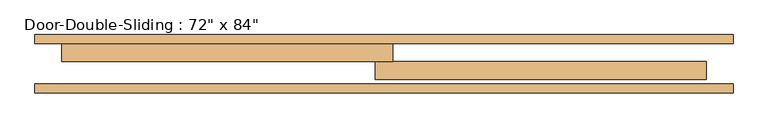
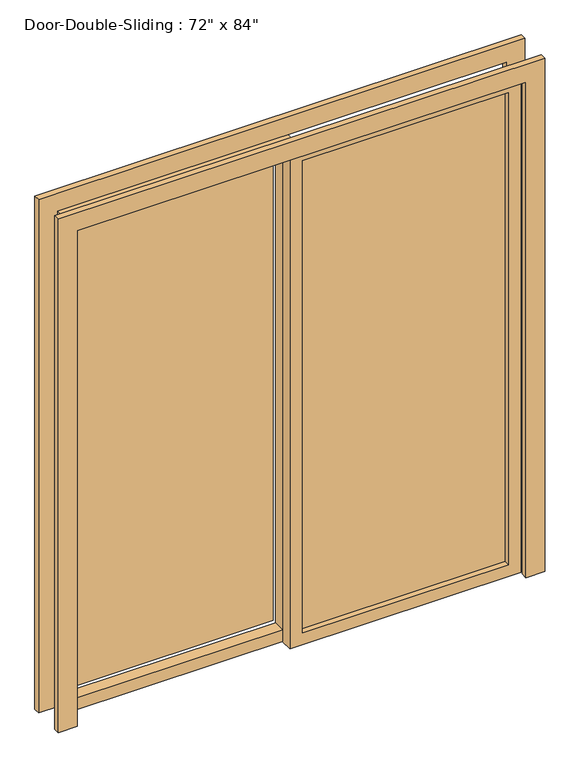
"""IFC4 building model written with IfcOpenShell, lengths in millimetres: door geometry."""

from ifc_helpers import new_model, si_unit, frame, origin, place, context, project, spatial, polyline, outline, extrude, source, transform, mapped, element, save


def door_166d4031(model_context):
    return source(origin(), model_context, "Body", "SweptSolid", [
        extrude(outline(polyline([(0.0, 990.6), (2209.8, 990.6), (2209.8, -990.6), (0.0, -990.6), (0.0, -914.4), (2133.6, -914.4), (2133.6, 914.4), (0.0, 914.4), (0.0, 990.6)])), frame((0.0, 184.15, 0.0), z_axis=(0.0, 1.0, 0.0), x_axis=(0.0, 0.0, 1.0)), (0.0, 0.0, 1.0), 25.4),
        extrude(outline(polyline([(0.0, -990.6), (0.0, -914.4), (2133.6, -914.4), (2133.6, 914.4), (0.0, 914.4), (0.0, 990.6), (2209.8, 990.6), (2209.8, -990.6), (0.0, -990.6)])), frame((0.0, 44.45, 0.0), z_axis=(0.0, 1.0, 0.0), x_axis=(0.0, 0.0, 1.0)), (0.0, 0.0, 1.0), 25.4),
        extrude(outline(polyline([(2133.6, 25.4), (2133.6, -914.4), (0.0, -914.4), (0.0, 25.4), (2133.6, 25.4)]), holes=[polyline([(2082.8, -25.4), (50.8, -25.4), (50.8, -863.6), (2082.8, -863.6), (2082.8, -25.4)])]), frame((0.0, 133.35, 0.0), z_axis=(0.0, 1.0, 0.0), x_axis=(0.0, 0.0, 1.0)), (0.0, 0.0, 1.0), 50.8),
        extrude(outline(polyline([(2133.6, -25.4), (0.0, -25.4), (0.0, 914.4), (2133.6, 914.4), (2133.6, -25.4)]), holes=[polyline([(2082.8, 25.4), (2082.8, 863.6), (50.8, 863.6), (50.8, 25.4), (2082.8, 25.4)])]), frame((0.0, 82.55, 0.0), z_axis=(0.0, 1.0, 0.0), x_axis=(0.0, 0.0, 1.0)), (0.0, 0.0, 1.0), 50.8),
        extrude(outline(polyline([(-25.4, 200.025), (-863.6, 200.025), (-863.6, 206.375), (-25.4, 206.375), (-25.4, 200.025)])), frame((0.0, 0.0, 50.8), z_axis=(0.0, 0.0, 1.0), x_axis=(1.0, 0.0, 0.0)), (0.0, 0.0, 1.0), 2032.0),
        extrude(outline(polyline([(25.4, 111.125), (863.6, 111.125), (863.6, 104.775), (25.4, 104.775), (25.4, 111.125)])), frame((0.0, 0.0, 50.8), z_axis=(0.0, 0.0, 1.0), x_axis=(1.0, 0.0, 0.0)), (0.0, 0.0, 1.0), 2032.0),
    ])


if __name__ == "__main__":
    model = new_model("IFC4")
    model_context = context("Model", 3, world=origin())
    ifc_project = project(units=[si_unit("LENGTHUNIT", "METRE", prefix="MILLI")], contexts=[model_context])
    site = spatial("IfcSite", under=ifc_project)
    building = spatial("IfcBuilding", under=site)
    placement = place(None, origin())
    door_shape = door_166d4031(model_context)
    element("IfcDoor", 1, ObjectType="Door-Double-Sliding : 72\" x 84\"", at=placement, inside=building, context=model_context, shape_type="MappedRepresentation", body=[
        mapped(door_shape, transform((0.0, 0.0, 0.0), x_axis=(1.0, 0.0, 0.0), y_axis=(0.0, 1.0, 0.0), z_axis=(0.0, 0.0, 1.0))),
    ])
    save(model, "model.ifc")

# Revit data of these elements
# Type "Door-Double-Sliding : 72\" x 84\""
#   Type Mark = "12"
#   Construction Type Id = "opn-d45"
#   Assembly Code = "C1020"
#   Analytic Construction = "Wood frame, double glass door "
#   Thickness = 0' - 2"
#   Thermal Resistance (R) = 1.8150 (h·ft²·°F)/BTU
#   Heat Transfer Coefficient (U) = 0.5510 BTU/(h·ft²·°F)
#   Height = 7' - 0"
#   Rail Width = 0' - 2"
#   Stiles = 0' - 2"
#   Trim Projection Ext = 0' - 1"
#   Trim Projection Int = 0' - 1"
#   Trim Width = 0' - 3"
#   Width = 6' - 0"
#   Define Thermal Properties by = 1
#   Glazing = Glass
#   Panel Material = Wood - Birch - Solid Stained Light Low Gloss
#   Trim Material = Paint - Sienna
#   Visual Light Transmittance = 0
#   Solar Heat Gain Coefficient = 0
#   Function = (empty or 0)
#   Wall Closure = (empty or 0)
# Element 1 (IfcDoor, "Door-Double-Sliding : 72\" x 84\"")
#   Materials on its faces: "Paint - Sienna", "Wood - Birch - Solid Stained Light Low Gloss", "Glass"
# Materials
#   "Glass": class "Glass", colour RGB 0 128 192, transparency 0.75, Description = "Soda Lime Glass", Cost = 0
#   "Wood - Birch - Solid Stained Light Low Gloss": class "Wood", colour RGB 210 159 95, transparency 0, Cost = 0
#   "Paint - Sienna": colour RGB 118 70 51, transparency 0, Cost = 0
